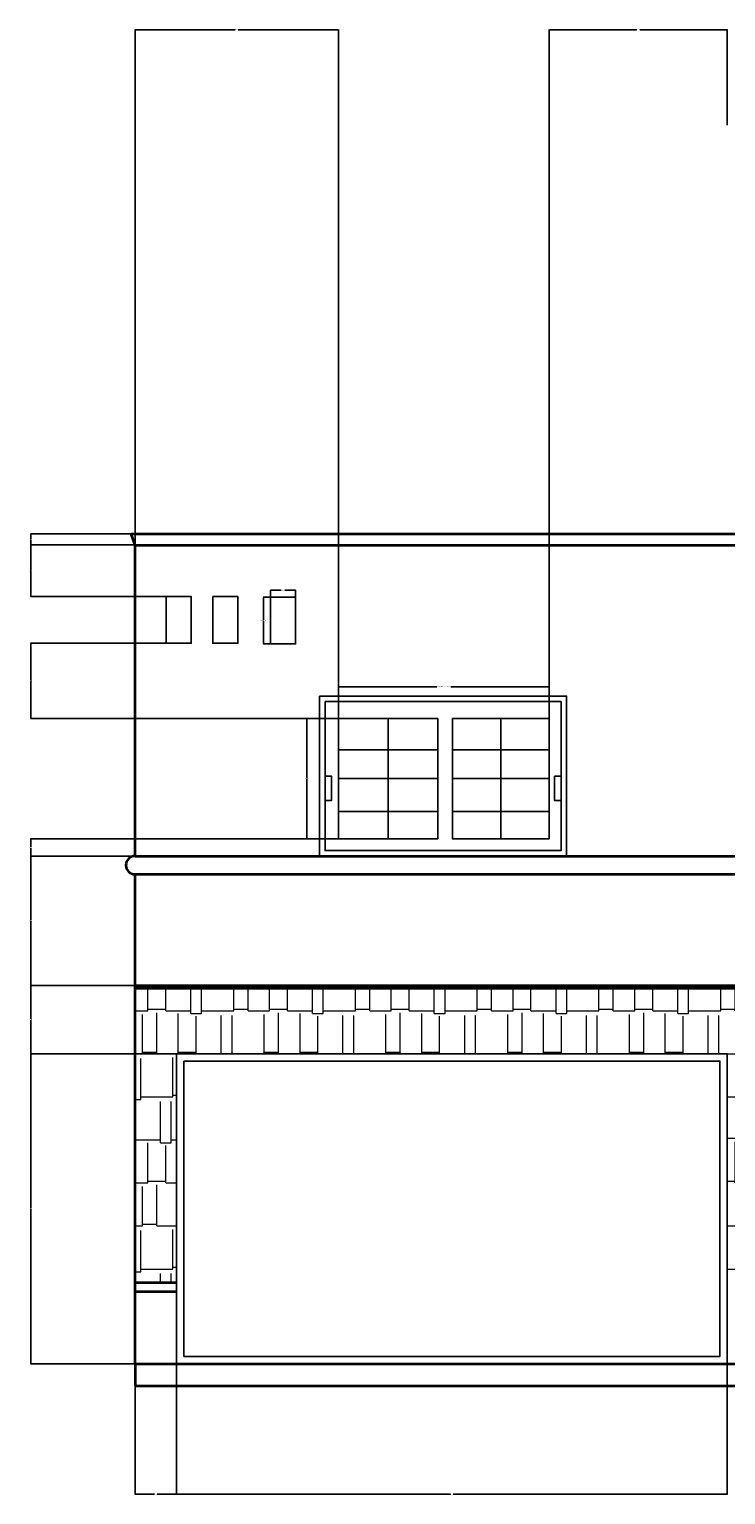
# Model space of a CAD drawing. Units: inches. Extents: x -73 to 2199, y -12 to 1583.
# Tile 1 of 3: x -73 to 686, y -12 to 1583. Entities that reach past the tile are written whole.
import ezdxf

# ---------------------------------------------------------------- set-up
doc = ezdxf.new("R2010")
doc.units = ezdxf.units.IN
doc.header["$MEASUREMENT"] = 0
for name, color, linetype, lineweight in [('A-ANNO-DIMS', 2, 'Continuous', 18), ('A-DOOR', 3, 'Continuous', 25), ('A-ELEV', 7, 'Continuous', 35), ('A-GLAZ', 4, 'Continuous', 25), ('A-ROOF', 7, 'Continuous', 35), ('A-WALL-PATT', 8, 'Continuous', 13)]:
    doc.layers.add(name, color=color, linetype=linetype, lineweight=lineweight)
doc.styles.get("Standard").update_dxf_attribs({"font": 'arial.ttf'})
doc.dimstyles.get("Standard").update_dxf_attribs({"dimtxt": 0.75, "dimasz": 0.18, "dimexe": 0.18, "dimexo": 0.0625, "dimgap": 0.09, "dimtad": 0, "dimtih": 1, "dimtoh": 1, "dimdec": 4, "dimzin": 0, "dimdsep": 46, "dimlunit": 4, "dimtxsty": 'Standard', "dimcen": 0.09, "dimadec": 0, "dimazin": 0, "dimtfac": 1, "dimtdec": 4, "dimtofl": 0, "dimtmove": 0, "dimatfit": 3, "dimfxl": 1, "dimtolj": 1, "dimtzin": 0, "dimarcsym": 0})

# ---------------------------------------------------------------- blocks, each defined once
blk = doc.blocks.new('WIN-CASEMENT-GRID')
for p, q in [((318.2, 767.7), (318.2, 833.2)), ((441.2, 833.2), (441.2, 702.2)), ((264.1, 799.1), (372.3, 799.1)), ((388.4, 799.1), (493.9, 799.1)), ((372.3, 767.7), (264.1, 767.7)), ((318.2, 767.7), (318.2, 702.2)), ((388.4, 767.7), (493.9, 767.7)), ((264.1, 731.8), (372.3, 731.8)), ((388.4, 731.8), (493.9, 731.8))]:
    blk.add_line(p, q)
for points in [[(264.1, 833.2), (372.3, 833.2), (372.3, 702.2), (264.1, 702.2)], [(388.4, 833.2), (493.9, 833.2), (493.9, 702.2), (388.4, 702.2)]]:
    blk.add_lwpolyline(points, close=True)
blk = doc.blocks.new('VENT-SMALL')
blk.add_lwpolyline([(76.5, 965.7), (103.9, 965.7), (103.9, 914.9), (76.5, 914.9)], close=True)
blk = doc.blocks.new('*D7')
at = {"layer": 'A-ANNO-DIMS', "color": 0, "lineweight": -2, "transparency": 16777216}
for p, q in [((190, 965), (182.3, 965)), ((182.4, 964.8), (182.4, 940.1)), ((182.4, 914.4), (182.4, 939.1)), ((190, 914.3), (182.3, 914.3))]:
    blk.add_line(p, q, dxfattribs=at)
at = {"layer": 'A-ANNO-DIMS', "color": 0, "transparency": 16777216}
for points in [[(182.4, 964.8), (182.5, 964.8), (182.4, 965)], [(182.4, 914.4), (182.5, 914.4), (182.4, 914.3)]]:
    blk.add_solid(points, dxfattribs=at)
at = {"layer": 'Defpoints', "color": 0, "transparency": 16777216}
for p in [(182.4, 965), (190, 965), (190, 914.3)]:
    blk.add_point(p, dxfattribs=at)
at = {"layer": 'A-ANNO-DIMS', "color": 0, "transparency": 16777216, "insert": (182.4, 939.6), "char_height": 0.75, "attachment_point": 5}
blk.add_mtext('\\A1;VENT 51 TYP.', dxfattribs=at)
blk = doc.blocks.new('*D8')
at = {"layer": 'A-ANNO-DIMS', "color": 0, "lineweight": -2, "transparency": 16777216}
for p, q in [((190, 965.1), (190, 972.8)), ((217.4, 965.1), (217.4, 972.8)), ((190.2, 972.6), (201.8, 972.6)), ((217.3, 972.6), (205.7, 972.6))]:
    blk.add_line(p, q, dxfattribs=at)
at = {"layer": 'A-ANNO-DIMS', "color": 0, "transparency": 16777216}
for points in [[(190.2, 972.6), (190.2, 972.6), (190, 972.6)], [(217.3, 972.6), (217.3, 972.6), (217.4, 972.6)]]:
    blk.add_solid(points, dxfattribs=at)
at = {"layer": 'Defpoints', "color": 0, "transparency": 16777216}
for p in [(190, 965), (217.4, 972.6), (217.4, 965)]:
    blk.add_point(p, dxfattribs=at)
at = {"layer": 'A-ANNO-DIMS', "color": 0, "transparency": 16777216, "insert": (203.7, 972.6), "char_height": 0.75, "attachment_point": 5}
blk.add_mtext('\\A1;27 TYP.', dxfattribs=at)
blk = doc.blocks.new('*D9')
at = {"layer": 'A-ANNO-DIMS', "color": 0, "lineweight": -2, "transparency": 16777216}
for p, q in [((264.1, 833.2), (264.1, 867.8)), ((264.2, 867.6), (371.3, 867.6)), ((493.8, 867.6), (386.7, 867.6)), ((493.9, 833.2), (493.9, 867.8))]:
    blk.add_line(p, q, dxfattribs=at)
at = {"layer": 'A-ANNO-DIMS', "color": 0, "transparency": 16777216}
for points in [[(264.2, 867.7), (264.2, 867.6), (264.1, 867.6)], [(493.8, 867.7), (493.8, 867.6), (493.9, 867.6)]]:
    blk.add_solid(points, dxfattribs=at)
at = {"layer": 'Defpoints', "color": 0, "transparency": 16777216}
for p in [(493.9, 867.6), (264.1, 833.2), (493.9, 833.2)]:
    blk.add_point(p, dxfattribs=at)
at = {"layer": 'A-ANNO-DIMS', "color": 0, "transparency": 16777216, "insert": (379, 867.6), "char_height": 0.75, "attachment_point": 5}
blk.add_mtext('\\A1;CASEMENT WINDOW 230 TYP.', dxfattribs=at)
blk = doc.blocks.new('*D10')
at = {"layer": 'A-ANNO-DIMS', "color": 0, "lineweight": -2, "transparency": 16777216}
for p, q in [((264, 833.2), (229.4, 833.2)), ((229.6, 833), (229.6, 768.2)), ((229.6, 702.4), (229.6, 767.2)), ((264, 702.2), (229.4, 702.2))]:
    blk.add_line(p, q, dxfattribs=at)
at = {"layer": 'A-ANNO-DIMS', "color": 0, "transparency": 16777216}
for points in [[(229.6, 833), (229.6, 833), (229.6, 833.2)], [(229.6, 702.4), (229.6, 702.4), (229.6, 702.2)]]:
    blk.add_solid(points, dxfattribs=at)
at = {"layer": 'Defpoints', "color": 0, "transparency": 16777216}
for p in [(229.6, 833.2), (264.1, 833.2), (264.1, 702.2)]:
    blk.add_point(p, dxfattribs=at)
at = {"layer": 'A-ANNO-DIMS', "color": 0, "transparency": 16777216, "insert": (229.6, 767.7), "char_height": 0.75, "attachment_point": 5}
blk.add_mtext('\\A1;131 TYP.', dxfattribs=at)
blk = doc.blocks.new('*D15')
at = {"layer": 'A-ANNO-DIMS', "color": 0, "lineweight": -2, "transparency": 16777216}
for p, q in [((42.6, 130.9), (42.6, -11.2)), ((87.8, 130.9), (87.8, -11.2)), ((42.8, -11), (63.9, -11)), ((87.6, -11), (66.6, -11))]:
    blk.add_line(p, q, dxfattribs=at)
at = {"layer": 'A-ANNO-DIMS', "color": 0, "transparency": 16777216}
for points in [[(42.8, -11), (42.8, -11.1), (42.6, -11)], [(87.6, -11), (87.6, -11.1), (87.8, -11)]]:
    blk.add_solid(points, dxfattribs=at)
at = {"layer": 'Defpoints', "color": 0, "transparency": 16777216}
for p in [(42.6, 131), (87.8, 131), (87.8, -11)]:
    blk.add_point(p, dxfattribs=at)
at = {"layer": 'A-ANNO-DIMS', "color": 0, "transparency": 16777216, "insert": (65.2, -11), "char_height": 0.75, "attachment_point": 5}
blk.add_mtext('\\A1;45.22', dxfattribs=at)
blk = doc.blocks.new('*D16')
at = {"layer": 'A-ANNO-DIMS', "color": 0, "lineweight": -2, "transparency": 16777216}
for p, q in [((87.8, 130.9), (87.8, -11.2)), ((687.8, 130.9), (687.8, -11.2)), ((88, -11), (386.4, -11)), ((687.6, -11), (389.2, -11))]:
    blk.add_line(p, q, dxfattribs=at)
at = {"layer": 'A-ANNO-DIMS', "color": 0, "transparency": 16777216}
for points in [[(88, -11), (88, -11.1), (87.8, -11)], [(687.6, -11), (687.6, -11.1), (687.8, -11)]]:
    blk.add_solid(points, dxfattribs=at)
at = {"layer": 'Defpoints', "color": 0, "transparency": 16777216}
for p in [(87.8, 131), (687.8, 131), (687.8, -11)]:
    blk.add_point(p, dxfattribs=at)
at = {"layer": 'A-ANNO-DIMS', "color": 0, "transparency": 16777216, "insert": (387.8, -11), "char_height": 0.75, "attachment_point": 5}
blk.add_mtext('\\A1;599.9', dxfattribs=at)
blk = doc.blocks.new('*D26')
at = {"layer": 'A-ANNO-DIMS', "color": 0, "lineweight": -2, "transparency": 16777216}
for p, q in [((42.6, 1022), (42.6, 1582.7)), ((42.8, 1582.6), (151.7, 1582.6)), ((263.9, 1582.6), (155, 1582.6)), ((264.1, 833.2), (264.1, 1582.7))]:
    blk.add_line(p, q, dxfattribs=at)
at = {"layer": 'A-ANNO-DIMS', "color": 0, "transparency": 16777216}
for points in [[(42.8, 1582.6), (42.8, 1582.5), (42.6, 1582.6)], [(263.9, 1582.6), (263.9, 1582.5), (264.1, 1582.6)]]:
    blk.add_solid(points, dxfattribs=at)
at = {"layer": 'Defpoints', "color": 0, "transparency": 16777216}
for p in [(264.1, 1582.6), (42.6, 1021.9), (264.1, 833.2)]:
    blk.add_point(p, dxfattribs=at)
at = {"layer": 'A-ANNO-DIMS', "color": 0, "transparency": 16777216, "insert": (153.3, 1582.6), "char_height": 0.75, "attachment_point": 5}
blk.add_mtext('\\A1;221.45', dxfattribs=at)
blk = doc.blocks.new('*D27')
at = {"layer": 'A-ANNO-DIMS', "color": 0, "lineweight": -2, "transparency": 16777216}
for p, q in [((493.9, 833.2), (493.9, 1582.7)), ((494.1, 1582.6), (589.2, 1582.6)), ((687.5, 1582.6), (592.4, 1582.6)), ((687.7, 1478.9), (687.7, 1582.7))]:
    blk.add_line(p, q, dxfattribs=at)
at = {"layer": 'A-ANNO-DIMS', "color": 0, "transparency": 16777216}
for points in [[(494.1, 1582.6), (494.1, 1582.5), (493.9, 1582.6)], [(687.5, 1582.6), (687.5, 1582.5), (687.7, 1582.6)]]:
    blk.add_solid(points, dxfattribs=at)
at = {"layer": 'Defpoints', "color": 0, "transparency": 16777216}
for p in [(687.7, 1582.6), (687.7, 1478.8), (493.9, 833.2)]:
    blk.add_point(p, dxfattribs=at)
at = {"layer": 'A-ANNO-DIMS', "color": 0, "transparency": 16777216, "insert": (590.8, 1582.6), "char_height": 0.75, "attachment_point": 5}
blk.add_mtext('\\A1;193.72', dxfattribs=at)
blk = doc.blocks.new('*D34')
at = {"layer": 'A-ANNO-DIMS', "color": 0, "lineweight": -2, "transparency": 16777216}
for p, q in [((87.8, 468.2), (-71.2, 468.2)), ((-71, 468), (-71, 300.1)), ((-71, 131.2), (-71, 299.1)), ((87.8, 131), (-71.2, 131))]:
    blk.add_line(p, q, dxfattribs=at)
at = {"layer": 'A-ANNO-DIMS', "color": 0, "transparency": 16777216}
for points in [[(-71.1, 468), (-71, 468), (-71, 468.2)], [(-71.1, 131.2), (-71, 131.2), (-71, 131)]]:
    blk.add_solid(points, dxfattribs=at)
at = {"layer": 'Defpoints', "color": 0, "transparency": 16777216}
for p in [(-71, 468.2), (87.8, 468.2), (87.8, 131)]:
    blk.add_point(p, dxfattribs=at)
at = {"layer": 'A-ANNO-DIMS', "color": 0, "transparency": 16777216, "insert": (-71, 299.6), "char_height": 0.75, "attachment_point": 5}
blk.add_mtext('\\A1;337.2', dxfattribs=at)
blk = doc.blocks.new('*D35')
at = {"layer": 'A-ANNO-DIMS', "color": 0, "lineweight": -2, "transparency": 16777216}
for p, q in [((42.6, 542.7), (-71.2, 542.7)), ((-71, 542.5), (-71, 505.9)), ((-71, 468.4), (-71, 505)), ((87.8, 468.2), (-71.2, 468.2))]:
    blk.add_line(p, q, dxfattribs=at)
at = {"layer": 'A-ANNO-DIMS', "color": 0, "transparency": 16777216}
for points in [[(-71.1, 542.5), (-71, 542.5), (-71, 542.7)], [(-71.1, 468.4), (-71, 468.4), (-71, 468.2)]]:
    blk.add_solid(points, dxfattribs=at)
at = {"layer": 'Defpoints', "color": 0, "transparency": 16777216}
for p in [(-71, 542.7), (42.6, 542.7), (87.8, 468.2)]:
    blk.add_point(p, dxfattribs=at)
at = {"layer": 'A-ANNO-DIMS', "color": 0, "transparency": 16777216, "insert": (-71, 505.5), "char_height": 0.75, "attachment_point": 5}
blk.add_mtext('\\A1;74.49', dxfattribs=at)
blk = doc.blocks.new('*D36')
at = {"layer": 'A-ANNO-DIMS', "color": 0, "lineweight": -2, "transparency": 16777216}
for p, q in [((42.6, 683.4), (-71.2, 683.4)), ((-71, 683.2), (-71, 613.5)), ((-71, 542.9), (-71, 612.6)), ((42.6, 542.7), (-71.2, 542.7))]:
    blk.add_line(p, q, dxfattribs=at)
at = {"layer": 'A-ANNO-DIMS', "color": 0, "transparency": 16777216}
for points in [[(-71.1, 683.2), (-71, 683.2), (-71, 683.4)], [(-71.1, 542.9), (-71, 542.9), (-71, 542.7)]]:
    blk.add_solid(points, dxfattribs=at)
at = {"layer": 'Defpoints', "color": 0, "transparency": 16777216}
for p in [(-71, 683.4), (42.6, 683.4), (42.6, 542.7)]:
    blk.add_point(p, dxfattribs=at)
at = {"layer": 'A-ANNO-DIMS', "color": 0, "transparency": 16777216, "insert": (-71, 613), "char_height": 0.75, "attachment_point": 5}
blk.add_mtext('\\A1;140.68', dxfattribs=at)
blk = doc.blocks.new('*D37')
at = {"layer": 'A-ANNO-DIMS', "color": 0, "lineweight": -2, "transparency": 16777216}
for p, q in [((264, 702.2), (-71.2, 702.2)), ((-71, 702), (-71, 693.3)), ((-71, 683.6), (-71, 692.3)), ((42.6, 683.4), (-71.2, 683.4))]:
    blk.add_line(p, q, dxfattribs=at)
at = {"layer": 'A-ANNO-DIMS', "color": 0, "transparency": 16777216}
for points in [[(-71.1, 702), (-71, 702), (-71, 702.2)], [(-71.1, 683.6), (-71, 683.6), (-71, 683.4)]]:
    blk.add_solid(points, dxfattribs=at)
at = {"layer": 'Defpoints', "color": 0, "transparency": 16777216}
for p in [(-71, 702.2), (264.1, 702.2), (42.6, 683.4)]:
    blk.add_point(p, dxfattribs=at)
at = {"layer": 'A-ANNO-DIMS', "color": 0, "transparency": 16777216, "insert": (-71, 692.8), "char_height": 0.75, "attachment_point": 5}
blk.add_mtext('\\A1;18.814', dxfattribs=at)
blk = doc.blocks.new('*D38')
at = {"layer": 'A-ANNO-DIMS', "color": 0, "lineweight": -2, "transparency": 16777216}
for p, q in [((76.4, 914.9), (-71.2, 914.9)), ((-71, 914.7), (-71, 874.5)), ((-71, 833.3), (-71, 873.6)), ((264, 833.2), (-71.2, 833.2))]:
    blk.add_line(p, q, dxfattribs=at)
at = {"layer": 'A-ANNO-DIMS', "color": 0, "transparency": 16777216}
for points in [[(-71.1, 914.7), (-71, 914.7), (-71, 914.9)], [(-71.1, 833.3), (-71, 833.3), (-71, 833.2)]]:
    blk.add_solid(points, dxfattribs=at)
at = {"layer": 'Defpoints', "color": 0, "transparency": 16777216}
for p in [(-71, 914.9), (76.5, 914.9), (264.1, 833.2)]:
    blk.add_point(p, dxfattribs=at)
at = {"layer": 'A-ANNO-DIMS', "color": 0, "transparency": 16777216, "insert": (-71, 874), "char_height": 0.75, "attachment_point": 5}
blk.add_mtext('\\A1;81.76', dxfattribs=at)
blk = doc.blocks.new('*D39')
at = {"layer": 'A-ANNO-DIMS', "color": 0, "lineweight": -2, "transparency": 16777216}
for p, q in [((42.6, 1021.9), (-71.2, 1021.9)), ((-71, 1021.7), (-71, 994.2)), ((-71, 965.8), (-71, 993.3)), ((76.4, 965.7), (-71.2, 965.7))]:
    blk.add_line(p, q, dxfattribs=at)
at = {"layer": 'A-ANNO-DIMS', "color": 0, "transparency": 16777216}
for points in [[(-71.1, 1021.7), (-71, 1021.7), (-71, 1021.9)], [(-71.1, 965.8), (-71, 965.8), (-71, 965.7)]]:
    blk.add_solid(points, dxfattribs=at)
at = {"layer": 'Defpoints', "color": 0, "transparency": 16777216}
for p in [(-71, 1021.9), (42.6, 1021.9), (76.5, 965.7)]:
    blk.add_point(p, dxfattribs=at)
at = {"layer": 'A-ANNO-DIMS', "color": 0, "transparency": 16777216, "insert": (-71, 993.8), "char_height": 0.75, "attachment_point": 5}
blk.add_mtext('\\A1;56.23', dxfattribs=at)
blk = doc.blocks.new('*D40')
at = {"layer": 'A-ANNO-DIMS', "color": 0, "lineweight": -2, "transparency": 16777216}
for p, q in [((38.3, 1033.9), (-71.2, 1033.9)), ((42.6, 1021.9), (-71.2, 1021.9)), ((-71, 1033.7), (-71, 1028.4)), ((-71, 1022.1), (-71, 1027.4))]:
    blk.add_line(p, q, dxfattribs=at)
at = {"layer": 'A-ANNO-DIMS', "color": 0, "transparency": 16777216}
for points in [[(-71.1, 1033.7), (-71, 1033.7), (-71, 1033.9)], [(-71.1, 1022.1), (-71, 1022.1), (-71, 1021.9)]]:
    blk.add_solid(points, dxfattribs=at)
at = {"layer": 'Defpoints', "color": 0, "transparency": 16777216}
for p in [(-71, 1033.9), (38.4, 1033.9), (42.6, 1021.9)]:
    blk.add_point(p, dxfattribs=at)
at = {"layer": 'A-ANNO-DIMS', "color": 0, "transparency": 16777216, "insert": (-71, 1027.9), "char_height": 0.75, "attachment_point": 5}
blk.add_mtext('\\A1;12', dxfattribs=at)

msp = doc.modelspace()

# ---------------------------------------------------------------- hatches: boundary and pattern name
at = {"layer": 'A-WALL-PATT'}
h = msp.add_hatch(dxfattribs=at)
h.set_pattern_fill('AR-RSHKE', color=256, scale=3.9)
h.paths.add_polyline_path([(736.9068, 539.7065), (42.6128, 539.7065), (42.6128, 419.0114), (42.6128, 219.3768), (87.8284, 219.3768), (87.8284, 468.215), (687.7643, 468.215), (687.7643, 219.3768), (736.9068, 219.3768)])
h.paths.add_polyline_path([(1665.5962, 450.9629), (1835.312, 450.9629), (1835.312, 194.4603), (1975.9662, 194.4603), (1975.9662, 539.7065), (1450.9568, 539.7065), (1450.9568, 194.4603), (1665.5962, 194.4603)])

# ---------------------------------------------------------------- linework, layer by layer
at = {"layer": 'A-DOOR'}
for points in [[(87.8284, 468.215), (687.7643, 468.215), (687.7643, 131.0114), (87.8284, 131.0114)], [(95.8284, 460.215), (679.7643, 460.215), (679.7643, 139.0114), (95.8284, 139.0114)]]:
    msp.add_lwpolyline(points, close=True, dxfattribs=at)
at = {"layer": 'A-ELEV'}
for p, q in [((42.6128, 1033.8877), (736.9068, 1033.8877)), ((42.6128, 683.3913), (42.6128, 1021.8877)), ((42.6128, 1021.8877), (736.9068, 1021.8877)), ((42.6128, 683.3913), (736.9068, 683.3913)), ((42.6128, 542.7065), (42.6128, 663.5939)), ((42.6128, 663.5939), (736.9068, 663.5939)), ((42.6128, 419.0114), (42.6128, 542.7065)), ((42.6128, 542.7065), (736.9068, 542.7065)), ((42.6128, 539.7065), (736.9068, 539.7065)), ((42.6128, 131.0114), (42.6128, 419.0114)), ((42.6128, 219.3768), (87.8284, 219.3768)), ((42.6128, 209.5972), (87.8284, 209.5972)), ((42.6128, 209.5972), (87.8284, 209.5972)), ((42.6128, 131.0114), (473.3051, 131.0114)), ((42.6128, 131.0114), (42.6128, 107.0114)), ((473.3051, 131.0114), (675.9771, 131.0114)), ((675.9771, 131.0114), (1134.5569, 131.0114)), ((42.6128, 107.0114), (473.3051, 107.0114)), ((473.3051, 107.0114), (677.7181, 107.0114)), ((677.7181, 107.0114), (1212.2414, 107.0114))]:
    msp.add_line(p, q, dxfattribs=at)
msp.add_arc((42.6128, 673.4926), 9.8987, 90, 270, dxfattribs=at)
at = {"layer": 'A-GLAZ'}
for points in [[(243.6443, 857.422), (512.6416, 857.422), (512.6416, 683.3913), (243.6443, 683.3913)], [(249.6443, 851.422), (506.6416, 851.422), (506.6416, 689.3913), (249.6443, 689.3913)], [(249.6443, 770.4066), (256.5865, 770.4066), (256.5865, 743.7381), (249.6443, 743.7381)], [(499.6994, 770.4066), (506.6416, 770.4066), (506.6416, 743.7381), (499.6994, 743.7381)]]:
    msp.add_lwpolyline(points, close=True, dxfattribs=at)
at = {"layer": 'A-ROOF'}
for p, q in [((42.6128, 1021.8877), (38.4043, 1033.8877)), ((38.4043, 1033.8877), (42.6128, 1033.8877))]:
    msp.add_line(p, q, dxfattribs=at)

# ---------------------------------------------------------------- block references
at = {"layer": 'A-GLAZ'}
for name, p in [('VENT-SMALL', (0, 0)), ('VENT-SMALL', (50.7779, 0)), ('VENT-SMALL', (113.5822, -0.6676)), ('WIN-CASEMENT-GRID', (0, 0))]:
    msp.add_blockref(name, p, dxfattribs=at)

# ---------------------------------------------------------------- dimensions: what is measured, and where the dimension line sits
at = {"layer": 'A-ANNO-DIMS'}
for base, p1, p2, override, picture, middle in [((264.067, 1582.5669), (42.6128, 1021.8877), (264.067, 833.1626), {"dimdec": 2, "dimlfac": 1, "dimrnd": 0, "dimzin": 0, "dimdsep": 46, "dimlunit": 2}, '*D26', (153.3399, 1582.5669)), ((687.6523, 1582.5669), (493.9311, 833.1626), (687.6523, 1478.8169), {"dimdec": 2, "dimlfac": 1, "dimrnd": 0, "dimzin": 0, "dimdsep": 46, "dimlunit": 2}, '*D27', (590.7917, 1582.5669)), ((87.8284, -11.0496), (42.6128, 131.0114), (87.8284, 131.0114), {"dimdec": 2, "dimlfac": 1, "dimrnd": 0, "dimzin": 0, "dimdsep": 46, "dimlunit": 2}, '*D15', (65.2206, -11.0496)), ((687.7643, -11.0496), (87.8284, 131.0114), (687.7643, 131.0114), {"dimdec": 1, "dimlfac": 1, "dimrnd": 0, "dimzin": 0, "dimdsep": 46, "dimlunit": 2}, '*D16', (387.7963, -11.0496))]:
    dim = msp.add_linear_dim(base=base, p1=p1, p2=p2, dimstyle='Standard', override=override, dxfattribs=at)
    dim.commit()
    dim.dimension.update_dxf_attribs({"geometry": picture, "text_midpoint": middle})
for base, p1, p2, override, picture, middle in [((-71.0359, 1021.8877), (76.4589, 965.6565), (42.6128, 1021.8877), {"dimdec": 2, "dimlfac": 1, "dimrnd": 0, "dimzin": 0, "dimdsep": 46, "dimlunit": 2}, '*D39', (-71.0359, 993.7721)), ((-71.0359, 1033.8877), (42.6128, 1021.8877), (38.4043, 1033.8877), {"dimdec": 0, "dimlfac": 1, "dimrnd": 0, "dimzin": 0, "dimdsep": 46, "dimlunit": 2}, '*D40', (-71.0359, 1027.8877)), ((-71.0359, 914.9193), (264.067, 833.1626), (76.4589, 914.9193), {"dimdec": 2, "dimlfac": 1, "dimrnd": 0, "dimzin": 0, "dimdsep": 46, "dimlunit": 2}, '*D38', (-71.0359, 874.0409)), ((-71.03588, 702.2048), (42.61281, 683.39126), (264.06703, 702.2048), {"dimdec": 3, "dimlfac": 1, "dimrnd": 0, "dimzin": 0, "dimdsep": 46, "dimlunit": 2}, '*D37', (-71.03588, 692.79803)), ((-71.0359, 683.3913), (42.6128, 542.7065), (42.6128, 683.3913), {"dimdec": 2, "dimlfac": 1, "dimrnd": 0, "dimzin": 0, "dimdsep": 46, "dimlunit": 2}, '*D36', (-71.0359, 613.0489)), ((-71.0359, 542.7065), (87.8284, 468.215), (42.6128, 542.7065), {"dimdec": 2, "dimlfac": 1, "dimrnd": 0, "dimzin": 0, "dimdsep": 46, "dimlunit": 2}, '*D35', (-71.0359, 505.4608)), ((-71.0359, 468.215), (87.8284, 131.0114), (87.8284, 468.215), {"dimdec": 1, "dimlfac": 1, "dimrnd": 0, "dimzin": 0, "dimdsep": 46, "dimlunit": 2}, '*D34', (-71.0359, 299.6132))]:
    dim = msp.add_linear_dim(base=base, p1=p1, p2=p2, angle=90, dimstyle='Standard', override=override, dxfattribs=at)
    dim.commit()
    dim.dimension.update_dxf_attribs({"geometry": picture, "text_midpoint": middle})
for base, p1, p2, text, picture, middle in [((217.4345, 972.5995), (190.0412, 964.9889), (217.4345, 964.9889), '<> TYP.', '*D8', (203.7378, 972.5995)), ((493.9311, 867.6423), (264.067, 833.1626), (493.9311, 833.1626), 'CASEMENT WINDOW <> TYP.', '*D9', (378.9991, 867.6423))]:
    dim = msp.add_linear_dim(base=base, p1=p1, p2=p2, text=text, dimstyle='Standard', override={"dimdec": 0, "dimlfac": 1, "dimrnd": 0, "dimzin": 0, "dimdsep": 46, "dimlunit": 2}, dxfattribs=at)
    dim.commit()
    dim.dimension.update_dxf_attribs({"geometry": picture, "text_midpoint": middle})
for base, p1, p2, text, picture, middle in [((182.4306, 964.9889), (190.0412, 914.2517), (190.0412, 964.9889), 'VENT <> TYP.', '*D7', (182.4306, 939.6203)), ((229.5874, 833.1626), (264.067, 702.2048), (264.067, 833.1626), '<> TYP.', '*D10', (229.5874, 767.6837))]:
    dim = msp.add_linear_dim(base=base, p1=p1, p2=p2, angle=90, text=text, dimstyle='Standard', override={"dimdec": 0, "dimlfac": 1, "dimrnd": 0, "dimzin": 0, "dimdsep": 46, "dimlunit": 2}, dxfattribs=at)
    dim.commit()
    dim.dimension.update_dxf_attribs({"geometry": picture, "text_midpoint": middle})

doc.saveas('drawing.dxf')
